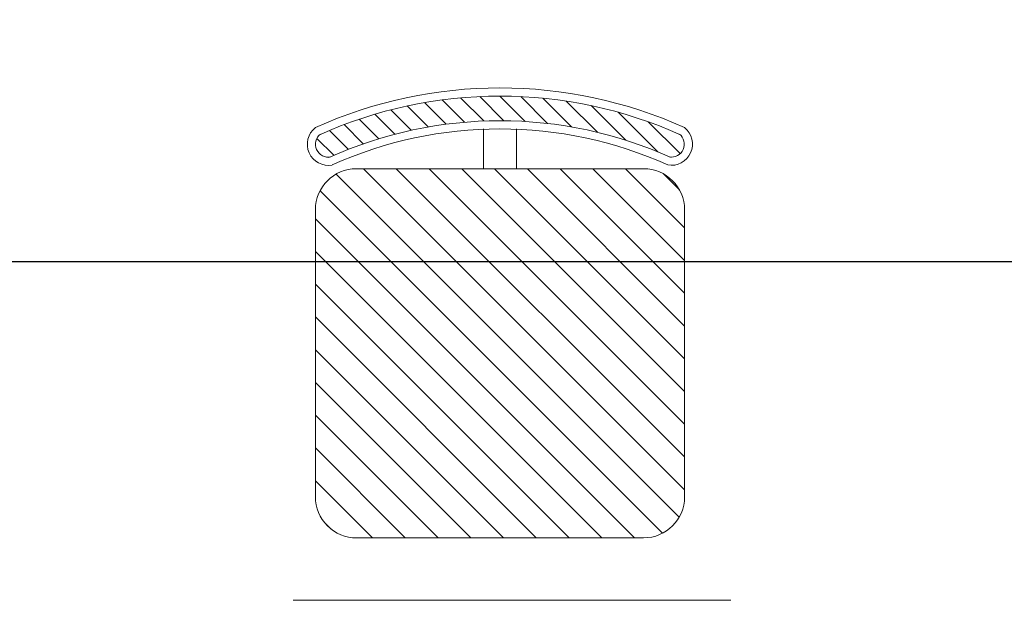
# Model space of a CAD drawing. Units: inches. Extents: x 375 to 1122, y 27 to 1069.
# Tile 148 of 155: x 705 to 747, y 917 to 941. Entities that reach past the tile are written whole.
import ezdxf

# ---------------------------------------------------------------- set-up
doc = ezdxf.new("R2010")
doc.units = ezdxf.units.IN
doc.layers.add('A-ANNO-DIMS', color=2, linetype='Continuous', lineweight=18)
doc.layers.add('Furniture', color=30, linetype='Continuous', lineweight=18)
doc.styles.get("Standard").update_dxf_attribs({"font": 'arial.ttf'})
doc.dimstyles.new('ISO-25', dxfattribs={"dimtxt": 12, "dimasz": 2.5, "dimexe": 1.5, "dimexo": 1.5, "dimtad": 1, "dimdec": 1, "dimlunit": 3, "dimtxsty": 'Standard', "dimblk": 'ARCHTICK', "dimcen": 2.5, "dimadec": 0, "dimazin": 0, "dimtfac": 1, "dimtdec": 1, "dimtmove": 0, "dimatfit": 3, "dimfxl": 1.5, "dimfxlon": 1, "dimarcsym": 0})

# ---------------------------------------------------------------- blocks, each defined once
blk = doc.blocks.new('A$C403C54AD')
for p, q in [((0.5449, 0.7957, -0.0006), (0.5449, 1.2611, -0.0006)), ((0.1295, 1.212, -0.0006), (0.4349, 1.212, -0.0006)), ((0.0859, 0.8629, -0.0006), (0.0859, 1.1683, -0.0006)), ((0.4785, 1.1683, -0.0006), (0.4785, 0.8629, -0.0006)), ((0.0859, 1.0331, -0.0006), (0.0436, 1.0331, -0.0006)), ((0.0859, 0.9982, -0.0006), (0.0436, 0.9982, -0.0006)), ((0.304, 0.8193, -0.0006), (0.1295, 0.8193, -0.0006)), ((0.4349, 0.8193, -0.0006), (0.304, 0.8193, -0.0006))]:
    blk.add_line(p, q)
at = {"ltscale": 0.05}
for p, q in [((0.0699, 1.2072, -0.0006), (0.0361, 1.1733, -0.0006)), ((0.4273, 1.212, -0.0006), (0.0859, 0.8705, -0.0006)), ((0.3925, 1.212, -0.0006), (0.0859, 0.9053, -0.0006)), ((0.3576, 1.212, -0.0006), (0.0859, 0.9402, -0.0006)), ((0.3228, 1.212, -0.0006), (0.0859, 0.975, -0.0006)), ((0.288, 1.212, -0.0006), (0.0859, 1.0098, -0.0006)), ((0.2532, 1.212, -0.0006), (0.0859, 1.0447, -0.0006)), ((0.2183, 1.212, -0.0006), (0.0859, 1.0795, -0.0006)), ((0.1835, 1.212, -0.0006), (0.0859, 1.1143, -0.0006)), ((0.1487, 1.212, -0.0006), (0.0859, 1.1491, -0.0006)), ((0.1084, 1.2065, -0.0006), (0.0913, 1.1894, -0.0006)), ((0.4564, 1.2063, -0.0006), (0.0916, 0.8414, -0.0006)), ((0.068, 1.1835, -0.0006), (0.0259, 1.1414, -0.0006)), ((0.4736, 1.1886, -0.0006), (0.1093, 0.8243, -0.0006)), ((0.4785, 1.1587, -0.0006), (0.1391, 0.8193, -0.0006)), ((0.0556, 1.1493, -0.0006), (0.0189, 1.1126, -0.0006)), ((0.4785, 1.1239, -0.0006), (0.1739, 0.8193, -0.0006)), ((0.0472, 1.1192, -0.0006), (0.014, 1.086, -0.0006)), ((0.0415, 1.0917, -0.0006), (0.0109, 1.0612, -0.0006)), ((0.4785, 1.0891, -0.0006), (0.2088, 0.8193, -0.0006)), ((0.0378, 1.0663, -0.0006), (0.0092, 1.0377, -0.0006)), ((0.4785, 1.0542, -0.0006), (0.2436, 0.8193, -0.0006)), ((0.0357, 1.0424, -0.0006), (0.0087, 1.0154, -0.0006)), ((0.0349, 1.0198, -0.0006), (0.0092, 0.9941, -0.0006)), ((0.4785, 1.0194, -0.0006), (0.2784, 0.8193, -0.0006)), ((0.0352, 0.9984, -0.0006), (0.0106, 0.9737, -0.0006)), ((0.4785, 0.9846, -0.0006), (0.3133, 0.8193, -0.0006)), ((0.0365, 0.9779, -0.0006), (0.0128, 0.9542, -0.0006)), ((0.0386, 0.9582, -0.0006), (0.0157, 0.9353, -0.0006)), ((0.4785, 0.9497, -0.0006), (0.3481, 0.8193, -0.0006)), ((0.0415, 0.9394, -0.0006), (0.0192, 0.917, -0.0006)), ((0.0451, 0.9212, -0.0006), (0.0234, 0.8994, -0.0006)), ((0.4785, 0.9149, -0.0006), (0.3829, 0.8193, -0.0006)), ((0.0493, 0.9036, -0.0006), (0.0281, 0.8824, -0.0006)), ((0.0541, 0.8867, -0.0006), (0.0333, 0.8658, -0.0006)), ((0.4785, 0.8801, -0.0006), (0.4177, 0.8193, -0.0006)), ((0.0595, 0.8702, -0.0006), (0.039, 0.8498, -0.0006)), ((0.0653, 0.8543, -0.0006), (0.0452, 0.8342, -0.0006)), ((0.0717, 0.8389, -0.0006), (0.0537, 0.8209, -0.0006)), ((0.4692, 0.8359, -0.0006), (0.4619, 0.8287, -0.0006))]:
    blk.add_line(p, q, dxfattribs=at)
for centre, radius, start, end in [((0.0598, 1.1978, -0.0006), 0.0225, 350.3316, 141.1036), ((0.4774, 1.0156, -0.0006), 0.4774, 155.7176, 204.2824), ((0.4774, 1.0156, -0.0006), 0.4687, 155.7176, 204.2824), ((0.0598, 1.1978, -0.0006), 0.0138, 350.3316, 141.1036), ((0.1295, 1.1683, -0.0006), 0.0436, 90, 180), ((0.4349, 1.1683, -0.0006), 0.0436, 0, 90), ((0.4774, 1.0156, -0.0006), 0.4425, 155.7176, 204.2824), ((0.4774, 1.0156, -0.0006), 0.4338, 155.7176, 204.2824), ((0.1295, 0.8629, -0.0006), 0.0436, 180, 270), ((0.4349, 0.8629, -0.0006), 0.0436, 270, 0), ((0.0599, 0.8332, -0.0006), 0.0225, 218.3306, 10.2342), ((0.0599, 0.8332, -0.0006), 0.0138, 218.3306, 10.2342)]:
    blk.add_arc(centre, radius, start, end)
blk = doc.blocks.new('_ArchTick')
at = {"color": 0, "linetype": 'ByBlock', "const_width": 0.15}
blk.add_lwpolyline([(-0.5, -0.5), (0.5, 0.5)], dxfattribs=at)
blk = doc.blocks.new('*D73')
at = {"layer": 'A-ANNO-DIMS', "color": 0, "lineweight": -2, "transparency": 16777216}
for p, q in [((686.757, 932.428), (686.757, 929.428)), ((770.757, 932.428), (770.757, 929.428)), ((686.757, 930.928), (770.757, 930.928)), ((770.757, 930.928), (987.61, 930.928))]:
    blk.add_line(p, q, dxfattribs=at)
at = {"layer": 'Defpoints', "color": 0, "transparency": 16777216}
for p in [(686.757, 943.528), (770.757, 943.528), (770.757, 930.928)]:
    blk.add_point(p, dxfattribs=at)
at = {"layer": 'A-ANNO-DIMS', "color": 0, "lineweight": -2, "transparency": 16777216, "xscale": 2.5, "yscale": 2.5, "zscale": 2.5, "rotation": 180}
blk.add_blockref('_ArchTick', (686.757, 930.928), dxfattribs=at)
at = {"layer": 'A-ANNO-DIMS', "color": 0, "lineweight": -2, "transparency": 16777216, "xscale": 2.5, "yscale": 2.5, "zscale": 2.5}
blk.add_blockref('_ArchTick', (770.757, 930.928), dxfattribs=at)
at = {"layer": 'A-ANNO-DIMS', "color": 0, "transparency": 16777216, "insert": (880.433, 937.757), "char_height": 12, "attachment_point": 5}
blk.add_mtext('2-PANEL SLIDER 7\'-0" TYP.', dxfattribs=at)
blk = doc.blocks.new('*D88')
at = {"layer": 'A-ANNO-DIMS', "color": 0, "lineweight": -2, "transparency": 16777216}
for p, q in [((731.007, 1052.528), (731.007, 1055.528)), ((854.007, 1052.528), (854.007, 1055.528)), ((731.007, 1054.028), (854.007, 1054.028))]:
    blk.add_line(p, q, dxfattribs=at)
at = {"layer": 'Defpoints', "color": 0, "transparency": 16777216}
for p in [(854.007, 1054.028), (731.007, 502.528), (854.007, 502.528)]:
    blk.add_point(p, dxfattribs=at)
at = {"layer": 'A-ANNO-DIMS', "color": 0, "lineweight": -2, "transparency": 16777216, "xscale": 2.5, "yscale": 2.5, "zscale": 2.5, "rotation": 180}
blk.add_blockref('_ArchTick', (731.007, 1054.028), dxfattribs=at)
at = {"layer": 'A-ANNO-DIMS', "color": 0, "lineweight": -2, "transparency": 16777216, "xscale": 2.5, "yscale": 2.5, "zscale": 2.5}
blk.add_blockref('_ArchTick', (854.007, 1054.028), dxfattribs=at)
at = {"layer": 'A-ANNO-DIMS', "color": 0, "transparency": 16777216, "insert": (792.507, 1060.784), "char_height": 12, "attachment_point": 5}
blk.add_mtext('10\'-3"', dxfattribs=at)
blk = doc.blocks.new('*D91')
at = {"layer": 'A-ANNO-DIMS', "color": 0, "lineweight": -2, "transparency": 16777216}
for p, q in [((728.007, 1052.528), (728.007, 1055.528)), ((788.007, 1052.528), (788.007, 1055.528)), ((728.007, 1054.028), (788.007, 1054.028))]:
    blk.add_line(p, q, dxfattribs=at)
at = {"layer": 'Defpoints', "color": 0, "transparency": 16777216}
for p in [(788.007, 1054.028), (728.007, 774.028), (788.007, 774.028)]:
    blk.add_point(p, dxfattribs=at)
at = {"layer": 'A-ANNO-DIMS', "color": 0, "lineweight": -2, "transparency": 16777216, "xscale": 2.5, "yscale": 2.5, "zscale": 2.5, "rotation": 180}
blk.add_blockref('_ArchTick', (728.007, 1054.028), dxfattribs=at)
at = {"layer": 'A-ANNO-DIMS', "color": 0, "lineweight": -2, "transparency": 16777216, "xscale": 2.5, "yscale": 2.5, "zscale": 2.5}
blk.add_blockref('_ArchTick', (788.007, 1054.028), dxfattribs=at)
at = {"layer": 'A-ANNO-DIMS', "color": 0, "transparency": 16777216, "insert": (758.007, 1060.78), "char_height": 12, "attachment_point": 5}
blk.add_mtext('5\'-0"', dxfattribs=at)

msp = doc.modelspace()

# ---------------------------------------------------------------- block references
at = {"layer": 'Furniture', "xscale": 39.9918517141215, "yscale": 39.9918517141215, "zscale": 39.9918517141215, "rotation": 270}
msp.add_blockref('A$C403C54AD', (684.955, 938.316, 0.024), dxfattribs=at)

# ---------------------------------------------------------------- dimensions: what is measured, and where the dimension line sits
at = {"layer": 'A-ANNO-DIMS'}
for base, p1, p2, picture, middle in [((788.007, 1054.028), (728.007, 774.028), (788.007, 774.028), '*D91', (758.007, 1060.78)), ((854.007, 1054.028), (731.007, 502.528), (854.007, 502.528), '*D88', (792.507, 1060.784))]:
    dim = msp.add_linear_dim(base=base, p1=p1, p2=p2, dimstyle='ISO-25', override={"dimdec": 1, "dimlfac": 1, "dimrnd": 0, "dimzin": 1, "dimdsep": 46, "dimlunit": 4, "dimfrac": 2}, dxfattribs=at)
    dim.commit()
    dim.dimension.update_dxf_attribs({"geometry": picture, "text_midpoint": middle})
dim = msp.add_linear_dim(base=(770.757, 930.928), p1=(686.757, 943.528), p2=(770.757, 943.528), text='2-PANEL SLIDER <> TYP.', dimstyle='ISO-25', override={"dimdec": 1, "dimlfac": 1, "dimrnd": 0, "dimzin": 1, "dimdsep": 46, "dimlunit": 4, "dimfrac": 2}, dxfattribs=at)
dim.commit()
dim.dimension.update_dxf_attribs({"geometry": '*D73', "text_midpoint": (880.433, 937.757)})

doc.saveas('drawing.dxf')
